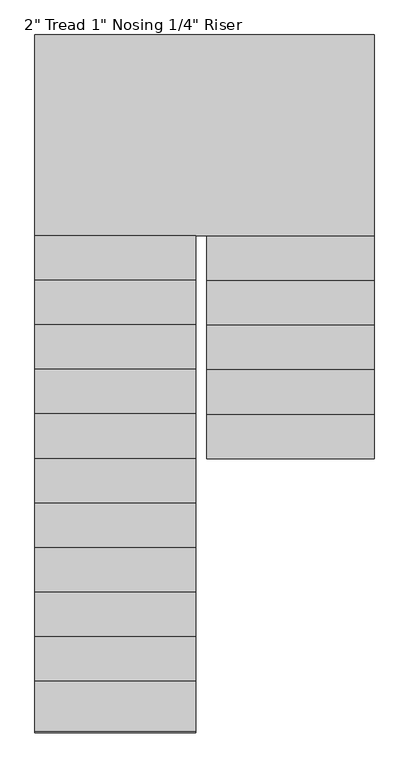
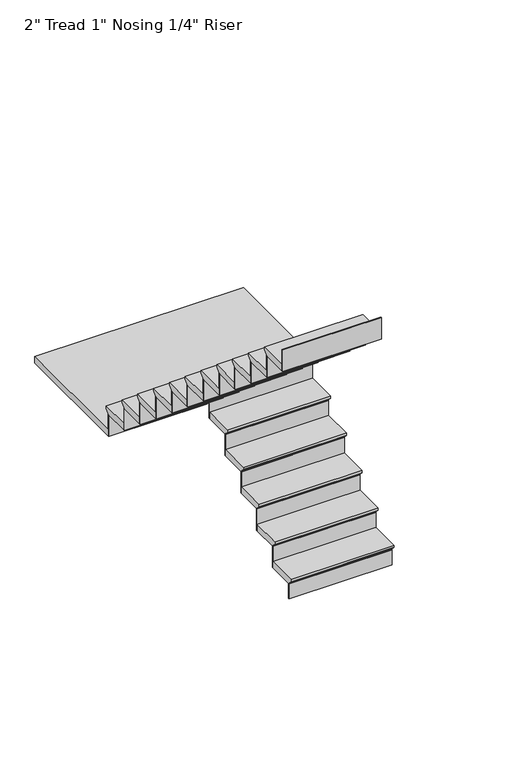
"""IFC4 building model written with IfcOpenShell, lengths in millimetres: stair flight geometry."""

from ifc_helpers import new_model, si_unit, origin, place, context, project, spatial, faceted_brep, source, transform, mapped, element, save


def stair_flight_8492ada7(model_context):
    return source(origin(), model_context, "Body", "Brep", [
        faceted_brep([(-3749.597125, 2714.6319226, 3198.2833333), (-3749.597125, 2714.6319226, 3217.3333333), (-4512.2136682, 2714.6319226, 3217.3333333), (-4512.2136682, 2714.6319226, 3198.2833333), (-3749.597125, 2740.0319226, 3172.8833333), (-4512.2136682, 2740.0319226, 3172.8833333), (-3749.597125, 2943.2319226, 3217.3333333), (-4512.2136682, 2943.2319226, 3217.3333333), (-4512.2136682, 2740.0319226, 3166.5333333), (-4512.2136682, 2943.2319226, 3166.5333333), (-3749.597125, 2943.2319226, 3166.5333333), (-3749.597125, 2740.0319226, 3166.5333333)], [[[0, 1, 2, 3]], [[4, 0, 3, 5]], [[2, 1, 6, 7]], [[8, 9, 10, 11]], [[2, 7, 9, 8, 5, 3]], [[8, 11, 4, 5]], [[6, 1, 0, 4, 11, 10]], [[7, 6, 10, 9]]]),
        faceted_brep([(-3749.597125, 2740.0319226, 3166.5333333), (-3749.597125, 2740.0319226, 3048.0), (-3749.597125, 2746.3819226, 3048.0), (-3749.597125, 2746.3819226, 3166.5333333), (-4512.2136682, 2740.0319226, 3166.5333333), (-4512.2136682, 2746.3819226, 3166.5333333), (-4512.2136682, 2746.3819226, 3048.0), (-4512.2136682, 2740.0319226, 3048.0)], [[[0, 1, 2, 3]], [[4, 5, 6, 7]], [[1, 0, 4, 7]], [[2, 1, 7, 6]], [[3, 2, 6, 5]], [[0, 3, 5, 4]]]),
        faceted_brep([(-3749.597125, 2943.2319226, 3335.8666667), (-3749.597125, 2943.2319226, 3166.5333333), (-3749.597125, 2949.5819226, 3166.5333333), (-3749.597125, 2949.5819226, 3335.8666667), (-4512.2136682, 2943.2319226, 3335.8666667), (-4512.2136682, 2949.5819226, 3335.8666667), (-4512.2136682, 2949.5819226, 3166.5333333), (-4512.2136682, 2943.2319226, 3166.5333333)], [[[0, 1, 2, 3]], [[4, 5, 6, 7]], [[1, 0, 4, 7]], [[2, 1, 7, 6]], [[3, 2, 6, 5]], [[0, 3, 5, 4]]]),
        faceted_brep([(-4512.2136682, 2917.8319226, 3386.6666667), (-3749.597125, 2917.8319226, 3386.6666667), (-3749.597125, 3146.4319226, 3386.6666667), (-4512.2136682, 3146.4319226, 3386.6666667), (-4512.2136682, 2943.2319226, 3335.8666667), (-4512.2136682, 3146.4319226, 3335.8666667), (-3749.597125, 3146.4319226, 3335.8666667), (-3749.597125, 2943.2319226, 3335.8666667), (-4512.2136682, 2943.2319226, 3342.2166667), (-4512.2136682, 2917.8319226, 3367.6166667), (-3749.597125, 2943.2319226, 3342.2166667), (-3749.597125, 2917.8319226, 3367.6166667)], [[[0, 1, 2, 3]], [[4, 5, 6, 7]], [[0, 3, 5, 4, 8, 9]], [[4, 7, 10, 8]], [[2, 1, 11, 10, 7, 6]], [[3, 2, 6, 5]], [[11, 1, 0, 9]], [[10, 11, 9, 8]]]),
        faceted_brep([(-3749.597125, 3146.4319226, 3505.2), (-3749.597125, 3146.4319226, 3335.8666667), (-3749.597125, 3152.7819226, 3335.8666667), (-3749.597125, 3152.7819226, 3505.2), (-4512.2136682, 3146.4319226, 3505.2), (-4512.2136682, 3152.7819226, 3505.2), (-4512.2136682, 3152.7819226, 3335.8666667), (-4512.2136682, 3146.4319226, 3335.8666667)], [[[0, 1, 2, 3]], [[4, 5, 6, 7]], [[1, 0, 4, 7]], [[2, 1, 7, 6]], [[3, 2, 6, 5]], [[0, 3, 5, 4]]]),
        faceted_brep([(-4512.2136682, 3121.0319226, 3556.0), (-3749.597125, 3121.0319226, 3556.0), (-3749.597125, 3349.6319226, 3556.0), (-4512.2136682, 3349.6319226, 3556.0), (-4512.2136682, 3146.4319226, 3505.2), (-4512.2136682, 3349.6319226, 3505.2), (-3749.597125, 3349.6319226, 3505.2), (-3749.597125, 3146.4319226, 3505.2), (-4512.2136682, 3146.4319226, 3511.55), (-4512.2136682, 3121.0319226, 3536.95), (-3749.597125, 3146.4319226, 3511.55), (-3749.597125, 3121.0319226, 3536.95)], [[[0, 1, 2, 3]], [[4, 5, 6, 7]], [[0, 3, 5, 4, 8, 9]], [[4, 7, 10, 8]], [[2, 1, 11, 10, 7, 6]], [[3, 2, 6, 5]], [[11, 1, 0, 9]], [[10, 11, 9, 8]]]),
        faceted_brep([(-3749.597125, 3349.6319226, 3674.5333333), (-3749.597125, 3349.6319226, 3505.2), (-3749.597125, 3355.9819226, 3505.2), (-3749.597125, 3355.9819226, 3674.5333333), (-4512.2136682, 3349.6319226, 3674.5333333), (-4512.2136682, 3355.9819226, 3674.5333333), (-4512.2136682, 3355.9819226, 3505.2), (-4512.2136682, 3349.6319226, 3505.2)], [[[0, 1, 2, 3]], [[4, 5, 6, 7]], [[1, 0, 4, 7]], [[2, 1, 7, 6]], [[3, 2, 6, 5]], [[0, 3, 5, 4]]]),
        faceted_brep([(-4512.2136682, 3324.2319226, 3725.3333333), (-3749.597125, 3324.2319226, 3725.3333333), (-3749.597125, 3552.8319226, 3725.3333333), (-4512.2136682, 3552.8319226, 3725.3333333), (-4512.2136682, 3349.6319226, 3674.5333333), (-4512.2136682, 3552.8319226, 3674.5333333), (-3749.597125, 3552.8319226, 3674.5333333), (-3749.597125, 3349.6319226, 3674.5333333), (-4512.2136682, 3349.6319226, 3680.8833333), (-4512.2136682, 3324.2319226, 3706.2833333), (-3749.597125, 3349.6319226, 3680.8833333), (-3749.597125, 3324.2319226, 3706.2833333)], [[[0, 1, 2, 3]], [[4, 5, 6, 7]], [[0, 3, 5, 4, 8, 9]], [[4, 7, 10, 8]], [[2, 1, 11, 10, 7, 6]], [[3, 2, 6, 5]], [[11, 1, 0, 9]], [[10, 11, 9, 8]]]),
        faceted_brep([(-3749.597125, 3552.8319226, 3843.8666667), (-3749.597125, 3552.8319226, 3674.5333333), (-3749.597125, 3559.1819226, 3674.5333333), (-3749.597125, 3559.1819226, 3843.8666667), (-4512.2136682, 3552.8319226, 3843.8666667), (-4512.2136682, 3559.1819226, 3843.8666667), (-4512.2136682, 3559.1819226, 3674.5333333), (-4512.2136682, 3552.8319226, 3674.5333333)], [[[0, 1, 2, 3]], [[4, 5, 6, 7]], [[1, 0, 4, 7]], [[2, 1, 7, 6]], [[3, 2, 6, 5]], [[0, 3, 5, 4]]]),
        faceted_brep([(-4512.2136682, 3527.4319226, 3894.6666667), (-3749.597125, 3527.4319226, 3894.6666667), (-3749.597125, 3756.0319226, 3894.6666667), (-4512.2136682, 3756.0319226, 3894.6666667), (-4512.2136682, 3552.8319226, 3843.8666667), (-4512.2136682, 3756.0319226, 3843.8666667), (-3749.597125, 3756.0319226, 3843.8666667), (-3749.597125, 3552.8319226, 3843.8666667), (-4512.2136682, 3552.8319226, 3850.2166667), (-4512.2136682, 3527.4319226, 3875.6166667), (-3749.597125, 3552.8319226, 3850.2166667), (-3749.597125, 3527.4319226, 3875.6166667)], [[[0, 1, 2, 3]], [[4, 5, 6, 7]], [[0, 3, 5, 4, 8, 9]], [[4, 7, 10, 8]], [[2, 1, 11, 10, 7, 6]], [[3, 2, 6, 5]], [[11, 1, 0, 9]], [[10, 11, 9, 8]]]),
        faceted_brep([(-3749.597125, 3756.0319226, 4013.2), (-3749.597125, 3756.0319226, 3843.8666667), (-3749.597125, 3762.3819226, 3843.8666667), (-3749.597125, 3762.3819226, 4013.2), (-4512.2136682, 3756.0319226, 4013.2), (-4512.2136682, 3762.3819226, 4013.2), (-4512.2136682, 3762.3819226, 3843.8666667), (-4512.2136682, 3756.0319226, 3843.8666667)], [[[0, 1, 2, 3]], [[4, 5, 6, 7]], [[1, 0, 4, 7]], [[2, 1, 7, 6]], [[3, 2, 6, 5]], [[0, 3, 5, 4]]]),
        faceted_brep([(-4563.0136682, 3705.2319226, 4064.0), (-4563.0136682, 3730.6319226, 4064.0), (-3749.597125, 3730.6319226, 4064.0), (-3749.597125, 4645.0319226, 4064.0), (-5295.0246464, 4645.0319226, 4064.0), (-5295.0246464, 3705.2319226, 4064.0), (-4563.0136682, 3730.6319226, 4013.2), (-4563.0136682, 3705.2319226, 4013.2), (-5295.0246464, 3705.2319226, 4013.2), (-5295.0246464, 4645.0319226, 4013.2), (-3749.597125, 4645.0319226, 4013.2), (-3749.597125, 3756.0319226, 4013.2), (-4512.2136682, 3756.0319226, 4013.2), (-4512.2136682, 3730.6319226, 4013.2), (-4512.2136682, 3730.6319226, 4044.95), (-3749.597125, 3730.6319226, 4044.95), (-4512.2136682, 3756.0319226, 4019.55), (-3749.597125, 3756.0319226, 4019.55)], [[[0, 1, 2, 3, 4, 5]], [[6, 7, 8, 9, 10, 11, 12, 13]], [[1, 0, 7, 6]], [[2, 1, 6, 13, 14, 15]], [[13, 12, 16, 14]], [[12, 11, 17, 16]], [[3, 2, 15, 17, 11, 10]], [[4, 3, 10, 9]], [[5, 4, 9, 8]], [[0, 5, 8, 7]], [[17, 15, 14, 16]]]),
        faceted_brep([(-5295.0246464, 3705.2319226, 4182.5333333), (-5295.0246464, 3705.2319226, 4013.2), (-5295.0246464, 3698.8819226, 4013.2), (-5295.0246464, 3698.8819226, 4182.5333333), (-4563.0136682, 3705.2319226, 4182.5333333), (-4563.0136682, 3698.8819226, 4182.5333333), (-4563.0136682, 3698.8819226, 4013.2), (-4563.0136682, 3705.2319226, 4013.2)], [[[0, 1, 2, 3]], [[4, 5, 6, 7]], [[1, 0, 4, 7]], [[2, 1, 7, 6]], [[3, 2, 6, 5]], [[0, 3, 5, 4]]]),
        faceted_brep([(-4563.0136682, 3730.6319226, 4233.3333333), (-5295.0246464, 3730.6319226, 4233.3333333), (-5295.0246464, 3502.0319226, 4233.3333333), (-4563.0136682, 3502.0319226, 4233.3333333), (-4563.0136682, 3705.2319226, 4182.5333333), (-4563.0136682, 3502.0319226, 4182.5333333), (-5295.0246464, 3502.0319226, 4182.5333333), (-5295.0246464, 3705.2319226, 4182.5333333), (-4563.0136682, 3705.2319226, 4188.8833333), (-4563.0136682, 3730.6319226, 4214.2833333), (-5295.0246464, 3705.2319226, 4188.8833333), (-5295.0246464, 3730.6319226, 4214.2833333)], [[[0, 1, 2, 3]], [[4, 5, 6, 7]], [[0, 3, 5, 4, 8, 9]], [[4, 7, 10, 8]], [[2, 1, 11, 10, 7, 6]], [[3, 2, 6, 5]], [[11, 1, 0, 9]], [[10, 11, 9, 8]]]),
        faceted_brep([(-5295.0246464, 3502.0319226, 4351.8666667), (-5295.0246464, 3502.0319226, 4182.5333333), (-5295.0246464, 3495.6819226, 4182.5333333), (-5295.0246464, 3495.6819226, 4351.8666667), (-4563.0136682, 3502.0319226, 4351.8666667), (-4563.0136682, 3495.6819226, 4351.8666667), (-4563.0136682, 3495.6819226, 4182.5333333), (-4563.0136682, 3502.0319226, 4182.5333333)], [[[0, 1, 2, 3]], [[4, 5, 6, 7]], [[1, 0, 4, 7]], [[2, 1, 7, 6]], [[3, 2, 6, 5]], [[0, 3, 5, 4]]]),
        faceted_brep([(-4563.0136682, 3527.4319226, 4402.6666667), (-5295.0246464, 3527.4319226, 4402.6666667), (-5295.0246464, 3298.8319226, 4402.6666667), (-4563.0136682, 3298.8319226, 4402.6666667), (-4563.0136682, 3502.0319226, 4351.8666667), (-4563.0136682, 3298.8319226, 4351.8666667), (-5295.0246464, 3298.8319226, 4351.8666667), (-5295.0246464, 3502.0319226, 4351.8666667), (-4563.0136682, 3502.0319226, 4358.2166667), (-4563.0136682, 3527.4319226, 4383.6166667), (-5295.0246464, 3502.0319226, 4358.2166667), (-5295.0246464, 3527.4319226, 4383.6166667)], [[[0, 1, 2, 3]], [[4, 5, 6, 7]], [[0, 3, 5, 4, 8, 9]], [[4, 7, 10, 8]], [[2, 1, 11, 10, 7, 6]], [[3, 2, 6, 5]], [[11, 1, 0, 9]], [[10, 11, 9, 8]]]),
        faceted_brep([(-5295.0246464, 3298.8319226, 4521.2), (-5295.0246464, 3298.8319226, 4351.8666667), (-5295.0246464, 3292.4819226, 4351.8666667), (-5295.0246464, 3292.4819226, 4521.2), (-4563.0136682, 3298.8319226, 4521.2), (-4563.0136682, 3292.4819226, 4521.2), (-4563.0136682, 3292.4819226, 4351.8666667), (-4563.0136682, 3298.8319226, 4351.8666667)], [[[0, 1, 2, 3]], [[4, 5, 6, 7]], [[1, 0, 4, 7]], [[2, 1, 7, 6]], [[3, 2, 6, 5]], [[0, 3, 5, 4]]]),
        faceted_brep([(-4563.0136682, 3324.2319226, 4572.0), (-5295.0246464, 3324.2319226, 4572.0), (-5295.0246464, 3095.6319226, 4572.0), (-4563.0136682, 3095.6319226, 4572.0), (-4563.0136682, 3298.8319226, 4521.2), (-4563.0136682, 3095.6319226, 4521.2), (-5295.0246464, 3095.6319226, 4521.2), (-5295.0246464, 3298.8319226, 4521.2), (-4563.0136682, 3298.8319226, 4527.55), (-4563.0136682, 3324.2319226, 4552.95), (-5295.0246464, 3298.8319226, 4527.55), (-5295.0246464, 3324.2319226, 4552.95)], [[[0, 1, 2, 3]], [[4, 5, 6, 7]], [[0, 3, 5, 4, 8, 9]], [[4, 7, 10, 8]], [[2, 1, 11, 10, 7, 6]], [[3, 2, 6, 5]], [[11, 1, 0, 9]], [[10, 11, 9, 8]]]),
        faceted_brep([(-5295.0246464, 3095.6319226, 4690.5333333), (-5295.0246464, 3095.6319226, 4521.2), (-5295.0246464, 3089.2819226, 4521.2), (-5295.0246464, 3089.2819226, 4690.5333333), (-4563.0136682, 3095.6319226, 4690.5333333), (-4563.0136682, 3089.2819226, 4690.5333333), (-4563.0136682, 3089.2819226, 4521.2), (-4563.0136682, 3095.6319226, 4521.2)], [[[0, 1, 2, 3]], [[4, 5, 6, 7]], [[1, 0, 4, 7]], [[2, 1, 7, 6]], [[3, 2, 6, 5]], [[0, 3, 5, 4]]]),
        faceted_brep([(-4563.0136682, 3121.0319226, 4741.3333333), (-5295.0246464, 3121.0319226, 4741.3333333), (-5295.0246464, 2892.4319226, 4741.3333333), (-4563.0136682, 2892.4319226, 4741.3333333), (-4563.0136682, 3095.6319226, 4690.5333333), (-4563.0136682, 2892.4319226, 4690.5333333), (-5295.0246464, 2892.4319226, 4690.5333333), (-5295.0246464, 3095.6319226, 4690.5333333), (-4563.0136682, 3095.6319226, 4696.8833333), (-4563.0136682, 3121.0319226, 4722.2833333), (-5295.0246464, 3095.6319226, 4696.8833333), (-5295.0246464, 3121.0319226, 4722.2833333)], [[[0, 1, 2, 3]], [[4, 5, 6, 7]], [[0, 3, 5, 4, 8, 9]], [[4, 7, 10, 8]], [[2, 1, 11, 10, 7, 6]], [[3, 2, 6, 5]], [[11, 1, 0, 9]], [[10, 11, 9, 8]]]),
        faceted_brep([(-5295.0246464, 2892.4319226, 4859.8666667), (-5295.0246464, 2892.4319226, 4690.5333333), (-5295.0246464, 2886.0819226, 4690.5333333), (-5295.0246464, 2886.0819226, 4859.8666667), (-4563.0136682, 2892.4319226, 4859.8666667), (-4563.0136682, 2886.0819226, 4859.8666667), (-4563.0136682, 2886.0819226, 4690.5333333), (-4563.0136682, 2892.4319226, 4690.5333333)], [[[0, 1, 2, 3]], [[4, 5, 6, 7]], [[1, 0, 4, 7]], [[2, 1, 7, 6]], [[3, 2, 6, 5]], [[0, 3, 5, 4]]]),
        faceted_brep([(-4563.0136682, 2917.8319226, 4910.6666667), (-5295.0246464, 2917.8319226, 4910.6666667), (-5295.0246464, 2689.2319226, 4910.6666667), (-4563.0136682, 2689.2319226, 4910.6666667), (-4563.0136682, 2892.4319226, 4859.8666667), (-4563.0136682, 2689.2319226, 4859.8666667), (-5295.0246464, 2689.2319226, 4859.8666667), (-5295.0246464, 2892.4319226, 4859.8666667), (-4563.0136682, 2892.4319226, 4866.2166667), (-4563.0136682, 2917.8319226, 4891.6166667), (-5295.0246464, 2892.4319226, 4866.2166667), (-5295.0246464, 2917.8319226, 4891.6166667)], [[[0, 1, 2, 3]], [[4, 5, 6, 7]], [[0, 3, 5, 4, 8, 9]], [[4, 7, 10, 8]], [[2, 1, 11, 10, 7, 6]], [[3, 2, 6, 5]], [[11, 1, 0, 9]], [[10, 11, 9, 8]]]),
        faceted_brep([(-5295.0246464, 2689.2319226, 5029.2), (-5295.0246464, 2689.2319226, 4859.8666667), (-5295.0246464, 2682.8819226, 4859.8666667), (-5295.0246464, 2682.8819226, 5029.2), (-4563.0136682, 2689.2319226, 5029.2), (-4563.0136682, 2682.8819226, 5029.2), (-4563.0136682, 2682.8819226, 4859.8666667), (-4563.0136682, 2689.2319226, 4859.8666667)], [[[0, 1, 2, 3]], [[4, 5, 6, 7]], [[1, 0, 4, 7]], [[2, 1, 7, 6]], [[3, 2, 6, 5]], [[0, 3, 5, 4]]]),
        faceted_brep([(-4563.0136682, 2714.6319226, 5080.0), (-5295.0246464, 2714.6319226, 5080.0), (-5295.0246464, 2486.0319226, 5080.0), (-4563.0136682, 2486.0319226, 5080.0), (-4563.0136682, 2689.2319226, 5029.2), (-4563.0136682, 2486.0319226, 5029.2), (-5295.0246464, 2486.0319226, 5029.2), (-5295.0246464, 2689.2319226, 5029.2), (-4563.0136682, 2689.2319226, 5035.55), (-4563.0136682, 2714.6319226, 5060.95), (-5295.0246464, 2689.2319226, 5035.55), (-5295.0246464, 2714.6319226, 5060.95)], [[[0, 1, 2, 3]], [[4, 5, 6, 7]], [[0, 3, 5, 4, 8, 9]], [[4, 7, 10, 8]], [[2, 1, 11, 10, 7, 6]], [[3, 2, 6, 5]], [[11, 1, 0, 9]], [[10, 11, 9, 8]]]),
        faceted_brep([(-5295.0246464, 2486.0319226, 5198.5333333), (-5295.0246464, 2486.0319226, 5029.2), (-5295.0246464, 2479.6819226, 5029.2), (-5295.0246464, 2479.6819226, 5198.5333333), (-4563.0136682, 2486.0319226, 5198.5333333), (-4563.0136682, 2479.6819226, 5198.5333333), (-4563.0136682, 2479.6819226, 5029.2), (-4563.0136682, 2486.0319226, 5029.2)], [[[0, 1, 2, 3]], [[4, 5, 6, 7]], [[1, 0, 4, 7]], [[2, 1, 7, 6]], [[3, 2, 6, 5]], [[0, 3, 5, 4]]]),
        faceted_brep([(-4563.0136682, 2511.4319226, 5249.3333333), (-5295.0246464, 2511.4319226, 5249.3333333), (-5295.0246464, 2282.8319226, 5249.3333333), (-4563.0136682, 2282.8319226, 5249.3333333), (-4563.0136682, 2486.0319226, 5198.5333333), (-4563.0136682, 2282.8319226, 5198.5333333), (-5295.0246464, 2282.8319226, 5198.5333333), (-5295.0246464, 2486.0319226, 5198.5333333), (-4563.0136682, 2486.0319226, 5204.8833333), (-4563.0136682, 2511.4319226, 5230.2833333), (-5295.0246464, 2486.0319226, 5204.8833333), (-5295.0246464, 2511.4319226, 5230.2833333)], [[[0, 1, 2, 3]], [[4, 5, 6, 7]], [[0, 3, 5, 4, 8, 9]], [[4, 7, 10, 8]], [[2, 1, 11, 10, 7, 6]], [[3, 2, 6, 5]], [[11, 1, 0, 9]], [[10, 11, 9, 8]]]),
        faceted_brep([(-5295.0246464, 2282.8319226, 5367.8666667), (-5295.0246464, 2282.8319226, 5198.5333333), (-5295.0246464, 2276.4819226, 5198.5333333), (-5295.0246464, 2276.4819226, 5367.8666667), (-4563.0136682, 2282.8319226, 5367.8666667), (-4563.0136682, 2276.4819226, 5367.8666667), (-4563.0136682, 2276.4819226, 5198.5333333), (-4563.0136682, 2282.8319226, 5198.5333333)], [[[0, 1, 2, 3]], [[4, 5, 6, 7]], [[1, 0, 4, 7]], [[2, 1, 7, 6]], [[3, 2, 6, 5]], [[0, 3, 5, 4]]]),
        faceted_brep([(-4563.0136682, 2308.2319226, 5418.6666667), (-5295.0246464, 2308.2319226, 5418.6666667), (-5295.0246464, 2079.6319226, 5418.6666667), (-4563.0136682, 2079.6319226, 5418.6666667), (-4563.0136682, 2282.8319226, 5367.8666667), (-4563.0136682, 2079.6319226, 5367.8666667), (-5295.0246464, 2079.6319226, 5367.8666667), (-5295.0246464, 2282.8319226, 5367.8666667), (-4563.0136682, 2282.8319226, 5374.2166667), (-4563.0136682, 2308.2319226, 5399.6166667), (-5295.0246464, 2282.8319226, 5374.2166667), (-5295.0246464, 2308.2319226, 5399.6166667)], [[[0, 1, 2, 3]], [[4, 5, 6, 7]], [[0, 3, 5, 4, 8, 9]], [[4, 7, 10, 8]], [[2, 1, 11, 10, 7, 6]], [[3, 2, 6, 5]], [[11, 1, 0, 9]], [[10, 11, 9, 8]]]),
        faceted_brep([(-5295.0246464, 2079.6319226, 5537.2), (-5295.0246464, 2079.6319226, 5367.8666667), (-5295.0246464, 2073.2819226, 5367.8666667), (-5295.0246464, 2073.2819226, 5537.2), (-4563.0136682, 2079.6319226, 5537.2), (-4563.0136682, 2073.2819226, 5537.2), (-4563.0136682, 2073.2819226, 5367.8666667), (-4563.0136682, 2079.6319226, 5367.8666667)], [[[0, 1, 2, 3]], [[4, 5, 6, 7]], [[1, 0, 4, 7]], [[2, 1, 7, 6]], [[3, 2, 6, 5]], [[0, 3, 5, 4]]]),
        faceted_brep([(-4563.0136682, 2105.0319226, 5588.0), (-5295.0246464, 2105.0319226, 5588.0), (-5295.0246464, 1876.4319226, 5588.0), (-4563.0136682, 1876.4319226, 5588.0), (-4563.0136682, 2079.6319226, 5537.2), (-4563.0136682, 1876.4319226, 5537.2), (-5295.0246464, 1876.4319226, 5537.2), (-5295.0246464, 2079.6319226, 5537.2), (-4563.0136682, 2079.6319226, 5543.55), (-4563.0136682, 2105.0319226, 5568.95), (-5295.0246464, 2079.6319226, 5543.55), (-5295.0246464, 2105.0319226, 5568.95)], [[[0, 1, 2, 3]], [[4, 5, 6, 7]], [[0, 3, 5, 4, 8, 9]], [[4, 7, 10, 8]], [[2, 1, 11, 10, 7, 6]], [[3, 2, 6, 5]], [[11, 1, 0, 9]], [[10, 11, 9, 8]]]),
        faceted_brep([(-5295.0246464, 1876.4319226, 5706.5333333), (-5295.0246464, 1876.4319226, 5537.2), (-5295.0246464, 1870.0819226, 5537.2), (-5295.0246464, 1870.0819226, 5706.5333333), (-4563.0136682, 1876.4319226, 5706.5333333), (-4563.0136682, 1870.0819226, 5706.5333333), (-4563.0136682, 1870.0819226, 5537.2), (-4563.0136682, 1876.4319226, 5537.2)], [[[0, 1, 2, 3]], [[4, 5, 6, 7]], [[1, 0, 4, 7]], [[2, 1, 7, 6]], [[3, 2, 6, 5]], [[0, 3, 5, 4]]]),
        faceted_brep([(-4563.0136682, 1901.8319226, 5757.3333333), (-5295.0246464, 1901.8319226, 5757.3333333), (-5295.0246464, 1673.2319226, 5757.3333333), (-4563.0136682, 1673.2319226, 5757.3333333), (-4563.0136682, 1876.4319226, 5706.5333333), (-4563.0136682, 1673.2319226, 5706.5333333), (-5295.0246464, 1673.2319226, 5706.5333333), (-5295.0246464, 1876.4319226, 5706.5333333), (-4563.0136682, 1876.4319226, 5712.8833333), (-4563.0136682, 1901.8319226, 5738.2833333), (-5295.0246464, 1876.4319226, 5712.8833333), (-5295.0246464, 1901.8319226, 5738.2833333)], [[[0, 1, 2, 3]], [[4, 5, 6, 7]], [[0, 3, 5, 4, 8, 9]], [[4, 7, 10, 8]], [[2, 1, 11, 10, 7, 6]], [[3, 2, 6, 5]], [[11, 1, 0, 9]], [[10, 11, 9, 8]]]),
        faceted_brep([(-5295.0246464, 1673.2319226, 5875.8666667), (-5295.0246464, 1673.2319226, 5706.5333333), (-5295.0246464, 1666.8819226, 5706.5333333), (-5295.0246464, 1666.8819226, 5875.8666667), (-4563.0136682, 1673.2319226, 5875.8666667), (-4563.0136682, 1666.8819226, 5875.8666667), (-4563.0136682, 1666.8819226, 5706.5333333), (-4563.0136682, 1673.2319226, 5706.5333333)], [[[0, 1, 2, 3]], [[4, 5, 6, 7]], [[1, 0, 4, 7]], [[2, 1, 7, 6]], [[3, 2, 6, 5]], [[0, 3, 5, 4]]]),
        faceted_brep([(-4563.0136682, 1698.6319226, 5926.6666667), (-5295.0246464, 1698.6319226, 5926.6666667), (-5295.0246464, 1470.0319226, 5926.6666667), (-4563.0136682, 1470.0319226, 5926.6666667), (-4563.0136682, 1673.2319226, 5875.8666667), (-4563.0136682, 1470.0319226, 5875.8666667), (-5295.0246464, 1470.0319226, 5875.8666667), (-5295.0246464, 1673.2319226, 5875.8666667), (-4563.0136682, 1673.2319226, 5882.2166667), (-4563.0136682, 1698.6319226, 5907.6166667), (-5295.0246464, 1673.2319226, 5882.2166667), (-5295.0246464, 1698.6319226, 5907.6166667)], [[[0, 1, 2, 3]], [[4, 5, 6, 7]], [[0, 3, 5, 4, 8, 9]], [[4, 7, 10, 8]], [[2, 1, 11, 10, 7, 6]], [[3, 2, 6, 5]], [[11, 1, 0, 9]], [[10, 11, 9, 8]]]),
        faceted_brep([(-5295.0246464, 1470.0319226, 6045.2), (-5295.0246464, 1470.0319226, 5875.8666667), (-5295.0246464, 1463.6819226, 5875.8666667), (-5295.0246464, 1463.6819226, 6045.2), (-4563.0136682, 1470.0319226, 6045.2), (-4563.0136682, 1463.6819226, 6045.2), (-4563.0136682, 1463.6819226, 5875.8666667), (-4563.0136682, 1470.0319226, 5875.8666667)], [[[0, 1, 2, 3]], [[4, 5, 6, 7]], [[1, 0, 4, 7]], [[2, 1, 7, 6]], [[3, 2, 6, 5]], [[0, 3, 5, 4]]]),
    ])


if __name__ == "__main__":
    model = new_model("IFC4")
    model_context = context("Model", 3, world=origin())
    ifc_project = project(units=[si_unit("LENGTHUNIT", "METRE", prefix="MILLI")], contexts=[model_context])
    site = spatial("IfcSite", under=ifc_project)
    building = spatial("IfcBuilding", under=site)
    placement = place(None, origin())
    stair_flight_shape = stair_flight_8492ada7(model_context)
    element("IfcStairFlight", 1, ObjectType="2\" Tread 1\" Nosing 1/4\" Riser", at=placement, inside=building, context=model_context, shape_type="MappedRepresentation", body=[
        mapped(stair_flight_shape, transform((0.0, 0.0, 0.0), x_axis=(1.0, 0.0, 0.0), y_axis=(0.0, 1.0, 0.0), z_axis=(0.0, 0.0, 1.0))),
    ])
    save(model, "model.ifc")
